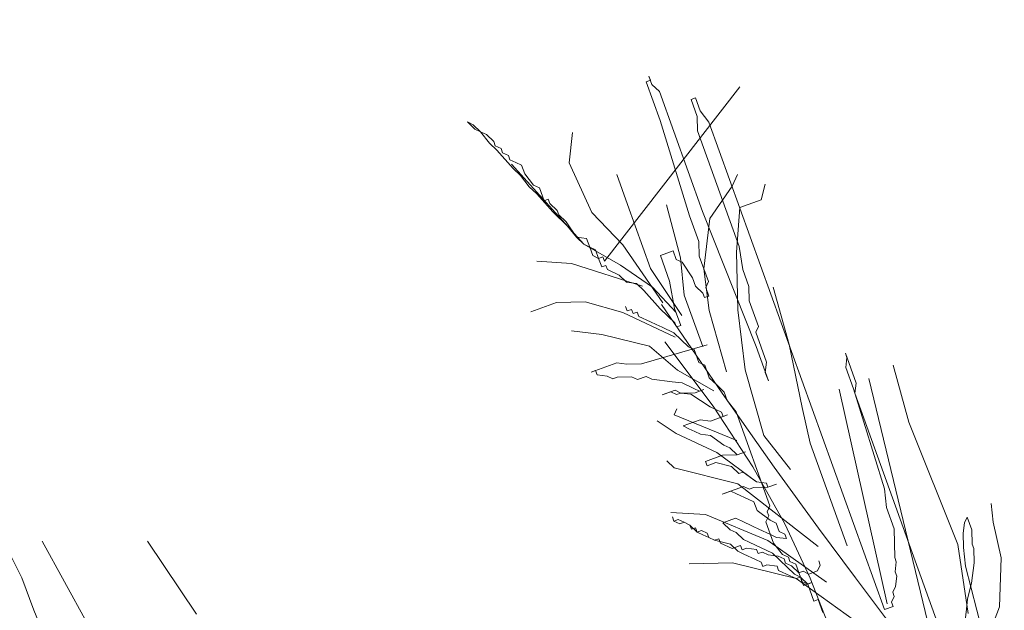
# Model space of a CAD drawing. Units: millimetres. Extents: x 595116 to 630915, y 909473 to 920225.
# Tile 88 of 134: x 629714.705 to 629720.901, y 919281.384 to 919285.103. Entities that reach past the tile are written whole.
import ezdxf

# ---------------------------------------------------------------- set-up
doc = ezdxf.new("R2010")
doc.units = ezdxf.units.MM
doc.layers.add('Dimension', color=3, linetype='Continuous', lineweight=18)
doc.layers.add('L-PLNT', color=85, linetype='Continuous', lineweight=13)
doc.styles.get("Standard").update_dxf_attribs({"font": 'arial.ttf'})
doc.dimstyles.new('ISO-25', dxfattribs={"dimtxt": 9, "dimasz": 6, "dimexe": 1.25, "dimexo": 0.625, "dimtad": 1, "dimlunit": 4, "dimtxsty": 'Standard', "dimcen": 2.5, "dimadec": 0, "dimazin": 0, "dimtfac": 1, "dimtmove": 0, "dimatfit": 3, "dimfxl": 1, "dimarcsym": 0})

# ---------------------------------------------------------------- blocks, each defined once
blk = doc.blocks.new('A$C4FB75ABC')
for p, q in [((2.238, 4.7104), (2.2329, 4.7248)), ((2.2329, 4.7248), (2.2354, 4.7176)), ((2.1583, 4.4143), (2.3852, 4.7066)), ((2.2354, 4.7176), (2.2283, 4.715)), ((2.2283, 4.715), (2.2515, 4.6504)), ((2.2504, 4.6987), (2.238, 4.7104)), ((2.3227, 4.4977), (2.2504, 4.6987)), ((2.3109, 4.688), (2.3037, 4.6854)), ((2.3037, 4.6854), (2.314, 4.6567)), ((2.3186, 4.6665), (2.3109, 4.688)), ((2.314, 4.6567), (2.3146, 4.6326)), ((2.3336, 4.6475), (2.3186, 4.6665)), ((1.9382, 4.6431), (1.9285, 4.6477)), ((1.9285, 4.6477), (1.9408, 4.6359)), ((1.9506, 4.6313), (1.9382, 4.6431)), ((2.2515, 4.6504), (2.3011, 4.49)), ((2.6279, 3.8295), (2.3336, 4.6475)), ((1.9408, 4.6359), (1.9506, 4.6313)), ((1.9603, 4.6267), (1.9506, 4.6313)), ((1.9506, 4.6313), (1.9655, 4.6124)), ((1.9726, 4.6149), (1.9603, 4.6267)), ((2.0989, 4.5793), (2.1049, 4.6301)), ((2.3146, 4.6326), (2.3843, 4.4389)), ((1.9655, 4.6124), (1.9778, 4.6006)), ((1.9752, 4.6078), (1.9726, 4.6149)), ((1.985, 4.6032), (1.9752, 4.6078)), ((1.9778, 4.6006), (2.0051, 4.5699)), ((1.9876, 4.596), (1.985, 4.6032)), ((1.9973, 4.5914), (1.9876, 4.596)), ((1.9999, 4.5842), (1.9973, 4.5914)), ((2.0097, 4.5796), (1.9999, 4.5842)), ((2.1238, 4.4424), (2.0025, 4.577)), ((2.0194, 4.575), (2.0097, 4.5796)), ((2.0246, 4.5607), (2.0194, 4.575)), ((2.137, 4.4958), (2.0989, 4.5793)), ((2.0051, 4.5699), (2.0174, 4.5581)), ((2.0174, 4.5581), (2.0323, 4.5391)), ((2.0395, 4.5417), (2.0246, 4.5607)), ((2.197, 4.5092), (2.1789, 4.5595)), ((2.3723, 4.5399), (2.3815, 4.5594)), ((2.0493, 4.5371), (2.0395, 4.5417)), ((2.4211, 4.5169), (2.4277, 4.5436)), ((2.0323, 4.5391), (2.0447, 4.5274)), ((2.0447, 4.5274), (2.0719, 4.4967)), ((2.057, 4.5156), (2.0493, 4.5371)), ((2.335, 4.486), (2.3723, 4.5399)), ((2.0642, 4.5182), (2.057, 4.5156)), ((2.0668, 4.511), (2.0642, 4.5182)), ((2.0791, 4.4992), (2.0668, 4.511)), ((2.2357, 4.4016), (2.197, 4.5092)), ((2.2859, 4.4197), (2.2621, 4.5084)), ((2.3852, 4.504), (2.4211, 4.5169)), ((2.0719, 4.4967), (2.0966, 4.4731)), ((2.0817, 4.4921), (2.0791, 4.4992)), ((2.094, 4.4803), (2.0817, 4.4921)), ((2.189, 4.4415), (2.137, 4.4958)), ((2.4125, 4.2707), (2.3227, 4.4977)), ((2.3797, 4.4291), (2.3852, 4.504)), ((2.1115, 4.4542), (2.094, 4.4803)), ((2.3011, 4.49), (2.3166, 4.4469)), ((2.325, 4.4013), (2.335, 4.486)), ((2.0966, 4.4731), (2.1115, 4.4542)), ((2.1238, 4.4424), (2.1115, 4.4542)), ((2.1115, 4.4542), (2.1284, 4.4522)), ((2.1336, 4.4378), (2.1238, 4.4424)), ((2.185, 4.4077), (2.1238, 4.4424)), ((2.1284, 4.4522), (2.1336, 4.4378)), ((2.2564, 4.3442), (2.189, 4.4415)), ((2.3166, 4.4469), (2.3172, 4.4228)), ((2.1388, 4.4235), (2.1336, 4.4378)), ((2.1336, 4.4378), (2.1434, 4.4332)), ((2.1434, 4.4332), (2.1485, 4.4189)), ((2.2736, 4.4314), (2.2521, 4.4237)), ((2.2788, 4.4171), (2.2736, 4.4314)), ((2.382, 4.3327), (2.3797, 4.4291)), ((2.3843, 4.4389), (2.3901, 4.4004)), ((2.1029, 4.4105), (2.0449, 4.414)), ((2.222, 4.3723), (2.1029, 4.4105)), ((2.1485, 4.4189), (2.1388, 4.4235)), ((2.1485, 4.4189), (2.1557, 4.4214)), ((2.1537, 4.4045), (2.1485, 4.4189)), ((2.1557, 4.4214), (2.1583, 4.4143)), ((2.2521, 4.4237), (2.2676, 4.3807)), ((2.2885, 4.4125), (2.2788, 4.4171)), ((2.2922, 4.3571), (2.2859, 4.4197)), ((2.306, 4.3864), (2.2885, 4.4125)), ((2.3172, 4.4228), (2.3327, 4.3798)), ((2.1609, 4.4071), (2.1537, 4.4045)), ((2.1634, 4.3999), (2.1609, 4.4071)), ((2.1829, 4.3907), (2.1634, 4.3999)), ((2.2389, 4.3703), (2.185, 4.4077)), ((2.2882, 4.3232), (2.2357, 4.4016)), ((2.3338, 4.3316), (2.325, 4.4013)), ((2.3901, 4.4004), (2.4004, 4.3717)), ((2.1953, 4.379), (2.1829, 4.3907)), ((2.2122, 4.3769), (2.1953, 4.379)), ((2.2245, 4.3652), (2.2122, 4.3769)), ((2.2676, 4.3807), (2.2759, 4.335)), ((2.3112, 4.372), (2.306, 4.3864)), ((2.3327, 4.3798), (2.3281, 4.37)), ((2.2518, 4.3344), (2.2245, 4.3652)), ((2.2785, 4.3278), (2.2389, 4.3703)), ((2.3235, 4.3603), (2.3112, 4.372)), ((2.3261, 4.3531), (2.3235, 4.3603)), ((2.3281, 4.37), (2.3333, 4.3557)), ((2.4004, 4.3717), (2.401, 4.3476)), ((2.4678, 4.2744), (2.4414, 4.3703)), ((2.0779, 4.3448), (2.0349, 4.3293)), ((2.1261, 4.346), (2.0779, 4.3448)), ((2.1893, 4.3282), (2.1261, 4.346)), ((2.3232, 4.271), (2.2922, 4.3571)), ((2.3333, 4.3557), (2.3261, 4.3531)), ((2.401, 4.3476), (2.4165, 4.3046)), ((2.277, 4.2868), (2.1893, 4.3282)), ((2.1938, 4.3379), (2.1964, 4.3307)), ((2.1964, 4.3307), (2.2036, 4.3333)), ((2.2036, 4.3333), (2.2062, 4.3261)), ((2.2062, 4.3261), (2.2134, 4.3287)), ((2.2134, 4.3287), (2.2159, 4.3215)), ((2.2641, 4.3227), (2.2518, 4.3344)), ((2.2538, 4.3417), (2.3557, 4.1924)), ((2.2759, 4.335), (2.2862, 4.3063)), ((2.3628, 4.2285), (2.3338, 4.3316)), ((2.3941, 4.2317), (2.382, 4.3327)), ((2.2159, 4.3215), (2.2354, 4.3124)), ((2.2354, 4.3124), (2.2452, 4.3078)), ((2.2765, 4.3109), (2.2641, 4.3227)), ((2.2791, 4.3037), (2.2765, 4.3109)), ((2.154, 4.2911), (2.1032, 4.2972)), ((2.2452, 4.3078), (2.255, 4.3032)), ((2.255, 4.3032), (2.2745, 4.294)), ((2.2745, 4.294), (2.2868, 4.2822)), ((2.2862, 4.3063), (2.2791, 4.3037)), ((2.4165, 4.3046), (2.4119, 4.2948)), ((2.4119, 4.2948), (2.43, 4.2446)), ((2.234, 4.2713), (2.154, 4.2911)), ((2.3407, 4.1707), (2.2593, 4.2788)), ((2.2868, 4.2822), (2.2991, 4.2704)), ((2.2202, 4.242), (2.3304, 4.2736)), ((2.2808, 4.2314), (2.234, 4.2713)), ((2.2991, 4.2704), (2.3089, 4.2658)), ((2.3089, 4.2658), (2.3166, 4.2443)), ((2.4331, 4.2133), (2.4125, 4.2707)), ((2.4896, 4.1688), (2.4678, 4.2744)), ((2.5803, 4.2095), (2.5622, 4.2597)), ((2.5622, 4.2597), (2.5648, 4.2526)), ((2.1362, 4.228), (2.1792, 4.2435)), ((2.1792, 4.2435), (2.1961, 4.2415)), ((2.3166, 4.2443), (2.3264, 4.2397)), ((2.43, 4.2446), (2.4279, 4.2276)), ((2.5648, 4.2526), (2.5628, 4.2356)), ((2.1434, 4.2306), (2.1362, 4.228)), ((2.1459, 4.2234), (2.1434, 4.2306)), ((2.1961, 4.2415), (2.2202, 4.242)), ((2.3419, 4.1967), (2.2808, 4.2314)), ((2.3264, 4.2397), (2.3341, 4.2182)), ((2.4257, 4.1214), (2.3941, 4.2317)), ((2.4279, 4.2276), (2.4331, 4.2133)), ((2.5628, 4.2356), (2.5757, 4.1997)), ((2.6686, 4.144), (2.6423, 4.2399)), ((2.1629, 4.2214), (2.1459, 4.2234)), ((2.1726, 4.2168), (2.1629, 4.2214)), ((2.1798, 4.2194), (2.1726, 4.2168)), ((2.2039, 4.22), (2.1798, 4.2194)), ((2.2136, 4.2154), (2.2039, 4.22)), ((2.228, 4.2205), (2.2136, 4.2154)), ((2.2377, 4.2159), (2.228, 4.2205)), ((2.2716, 4.2119), (2.2377, 4.2159)), ((2.2885, 4.2099), (2.2716, 4.2119)), ((2.308, 4.2007), (2.2885, 4.2099)), ((2.3341, 4.2182), (2.3465, 4.2064)), ((2.7169, 3.7399), (2.6018, 4.2172)), ((2.2552, 4.1898), (2.2768, 4.1975)), ((2.2696, 4.195), (2.2552, 4.1898)), ((2.2793, 4.1904), (2.2696, 4.195)), ((2.2768, 4.1975), (2.2865, 4.1929)), ((2.2865, 4.1929), (2.3106, 4.1935)), ((2.3178, 4.1961), (2.308, 4.2007)), ((2.3106, 4.1935), (2.325, 4.1987)), ((2.325, 4.1987), (2.3178, 4.1961)), ((2.3465, 4.2064), (2.3588, 4.1946)), ((2.3588, 4.1946), (2.364, 4.1803)), ((2.6325, 3.8393), (2.5516, 4.1992)), ((2.5757, 4.1997), (2.6279, 4.0321)), ((2.5783, 4.1926), (2.5803, 4.2095)), ((2.2865, 4.1929), (2.2793, 4.1904)), ((2.3034, 4.1909), (2.2865, 4.1929)), ((2.3353, 4.17), (2.3034, 4.1909)), ((2.3557, 4.1924), (2.443, 4.0685)), ((2.364, 4.1803), (2.3789, 4.1614)), ((2.8029, 3.5683), (2.5783, 4.1926)), ((2.2753, 4.1565), (2.2799, 4.1663)), ((2.345, 4.1654), (2.3353, 4.17)), ((2.4072, 4.0691), (2.3407, 4.1707)), ((2.3548, 4.1608), (2.345, 4.1654)), ((2.3574, 4.1536), (2.3548, 4.1608)), ((2.3789, 4.1614), (2.4357, 4.0035)), ((2.5031, 4.1088), (2.4896, 4.1688)), ((2.2785, 4.1252), (2.2466, 4.1462)), ((2.38, 4.1131), (2.2753, 4.1565)), ((2.2902, 4.1376), (2.3189, 4.1479)), ((2.3189, 4.1479), (2.3359, 4.1459)), ((2.3359, 4.1459), (2.3645, 4.1562)), ((2.3645, 4.1562), (2.3574, 4.1536)), ((2.7507, 3.9385), (2.6686, 4.144)), ((2.3, 4.133), (2.2902, 4.1376)), ((2.3098, 4.1284), (2.3, 4.133)), ((2.3195, 4.1238), (2.3098, 4.1284)), ((2.3468, 4.0931), (2.2785, 4.1252)), ((2.3364, 4.1218), (2.3195, 4.1238)), ((2.3585, 4.1054), (2.3364, 4.1218)), ((2.4704, 4.0646), (2.4257, 4.1214)), ((2.3683, 4.1008), (2.3585, 4.1054)), ((2.3806, 4.089), (2.3683, 4.1008)), ((2.5651, 3.9366), (2.5031, 4.1088)), ((2.275, 4.0672), (2.2627, 4.079)), ((2.3278, 4.0781), (2.3565, 4.0885)), ((2.3304, 4.071), (2.3278, 4.0781)), ((2.413, 4.044), (2.3468, 4.0931)), ((2.3565, 4.0885), (2.3806, 4.089)), ((2.3806, 4.089), (2.395, 4.0942)), ((2.395, 4.0942), (2.3806, 4.089)), ((2.3818, 4.0408), (2.275, 4.0672)), ((2.3448, 4.0761), (2.3304, 4.071)), ((2.3714, 4.0695), (2.3448, 4.0761)), ((2.3838, 4.0577), (2.3714, 4.0695)), ((2.4608, 3.9732), (2.4072, 4.0691)), ((2.443, 4.0685), (2.5171, 3.9664)), ((2.3909, 4.0603), (2.3838, 4.0577)), ((2.413, 4.044), (2.3909, 4.0603)), ((2.3557, 4.0233), (2.3915, 4.0362)), ((2.37, 4.0285), (2.3557, 4.0233)), ((2.3798, 4.0239), (2.37, 4.0285)), ((2.5169, 3.9354), (2.3818, 4.0408)), ((2.3915, 4.0362), (2.4013, 4.0316)), ((2.4013, 4.0316), (2.4084, 4.0342)), ((2.4084, 4.0342), (2.4325, 4.0348)), ((2.43, 4.0419), (2.413, 4.044)), ((2.4325, 4.0348), (2.43, 4.0419)), ((2.4325, 4.0348), (2.4469, 4.0399)), ((2.4469, 4.0399), (2.4325, 4.0348)), ((2.6279, 4.0321), (2.6311, 4.0008)), ((2.3993, 4.0147), (2.3798, 4.0239)), ((2.409, 4.0101), (2.3993, 4.0147)), ((2.4142, 3.9957), (2.409, 4.0101)), ((2.4363, 3.9794), (2.4142, 3.9957)), ((2.4357, 4.0035), (2.4311, 3.9937)), ((2.6311, 4.0008), (2.644, 3.965)), ((2.8101, 3.9761), (2.8069, 4.0074)), ((2.3275, 3.9889), (2.2696, 3.9923)), ((2.2748, 3.978), (2.2722, 3.9852)), ((2.2722, 3.9852), (2.2748, 3.978)), ((2.2748, 3.978), (2.2819, 3.9806)), ((2.2819, 3.9806), (2.2917, 3.976)), ((2.4323, 3.9455), (2.3275, 3.9889)), ((2.3568, 3.9751), (2.3783, 3.9828)), ((2.3783, 3.9828), (2.3881, 3.9782)), ((2.4337, 3.9866), (2.4291, 3.9768)), ((2.4311, 3.9937), (2.4337, 3.9866)), ((2.446, 3.9748), (2.4363, 3.9794)), ((2.7665, 3.9847), (2.7619, 3.975)), ((2.7742, 3.9632), (2.7665, 3.9847)), ((2.2845, 3.9734), (2.2748, 3.978)), ((2.2917, 3.976), (2.2845, 3.9734)), ((2.3014, 3.9714), (2.2917, 3.976)), ((2.2917, 3.976), (2.3014, 3.9714)), ((2.304, 3.9642), (2.3014, 3.9714)), ((2.3014, 3.9714), (2.3138, 3.9596)), ((2.3112, 3.9668), (2.304, 3.9642)), ((2.3138, 3.9596), (2.3112, 3.9668)), ((2.3691, 3.9633), (2.3568, 3.9751)), ((2.3789, 3.9587), (2.3691, 3.9633)), ((2.3881, 3.9782), (2.4076, 3.9691)), ((2.4076, 3.9691), (2.4173, 3.9645)), ((2.4173, 3.9645), (2.4368, 3.9553)), ((2.4291, 3.9768), (2.442, 3.9409)), ((2.4512, 3.9604), (2.446, 3.9748)), ((2.5035, 3.8821), (2.4608, 3.9732)), ((2.5171, 3.9664), (2.5794, 3.8826)), ((2.644, 3.965), (2.6451, 3.9167)), ((2.7619, 3.975), (2.7599, 3.958)), ((2.7748, 3.9391), (2.7742, 3.9632)), ((2.8236, 3.9161), (2.8101, 3.9761)), ((2.3209, 3.9622), (2.3138, 3.9596)), ((2.3138, 3.9596), (2.3235, 3.955)), ((2.3307, 3.9576), (2.3209, 3.9622)), ((2.3235, 3.955), (2.3333, 3.9504)), ((2.3333, 3.9504), (2.3307, 3.9576)), ((2.343, 3.9458), (2.3333, 3.9504)), ((2.3333, 3.9504), (2.343, 3.9458)), ((2.3502, 3.9484), (2.343, 3.9458)), ((2.343, 3.9458), (2.3697, 3.9392)), ((2.3528, 3.9412), (2.3502, 3.9484)), ((2.3912, 3.947), (2.3789, 3.9587)), ((2.401, 3.9424), (2.3912, 3.947)), ((2.4368, 3.9553), (2.4466, 3.9507)), ((2.4466, 3.9507), (2.4635, 3.9487)), ((2.4609, 3.9558), (2.4512, 3.9604)), ((2.4635, 3.9487), (2.4609, 3.9558)), ((2.7599, 3.958), (2.7605, 3.9339)), ((1.154, 3.9374), (1.1812, 3.8829)), ((1.2153, 3.9442), (1.2902, 3.808)), ((1.3924, 3.9442), (1.4742, 3.8217)), ((2.3723, 3.932), (2.3528, 3.9412)), ((2.3697, 3.9392), (2.3821, 3.9274)), ((2.3866, 3.9372), (2.3723, 3.932)), ((2.3892, 3.93), (2.3866, 3.9372)), ((2.3964, 3.9326), (2.3892, 3.93)), ((2.4133, 3.9306), (2.3964, 3.9326)), ((2.44, 3.924), (2.401, 3.9424)), ((2.4159, 3.9234), (2.4133, 3.9306)), ((2.5304, 3.8755), (2.4323, 3.9455)), ((2.442, 3.9409), (2.4569, 3.922)), ((2.7679, 3.8231), (2.7507, 3.9385)), ((2.7605, 3.9339), (2.7636, 3.9026)), ((2.7774, 3.9319), (2.7748, 3.9391)), ((2.778, 3.9078), (2.7774, 3.9319)), ((2.3821, 3.9274), (2.3918, 3.9228)), ((2.3918, 3.9228), (2.4113, 3.9137)), ((2.4113, 3.9137), (2.4211, 3.9091)), ((2.4231, 3.926), (2.4159, 3.9234)), ((2.4328, 3.9214), (2.4231, 3.926)), ((2.4498, 3.9194), (2.4328, 3.9214)), ((2.4523, 3.9122), (2.44, 3.924)), ((2.4595, 3.9148), (2.4498, 3.9194)), ((2.4569, 3.922), (2.4667, 3.9174)), ((2.4621, 3.9076), (2.4595, 3.9148)), ((2.4667, 3.9174), (2.4693, 3.9102)), ((2.6451, 3.9167), (2.6477, 3.9096)), ((2.8207, 3.834), (2.8236, 3.9161)), ((2.3729, 3.9079), (2.3006, 3.9062)), ((2.4796, 3.8815), (2.3729, 3.9079)), ((2.4211, 3.9091), (2.4237, 3.9019)), ((2.4237, 3.9019), (2.4308, 3.9045)), ((2.4308, 3.9045), (2.4478, 3.9025)), ((2.4478, 3.9025), (2.4503, 3.8953)), ((2.477, 3.8887), (2.4523, 3.9122)), ((2.4718, 3.903), (2.4621, 3.9076)), ((2.4693, 3.9102), (2.479, 3.9056)), ((2.4842, 3.8913), (2.4718, 3.903)), ((2.479, 3.9056), (2.4868, 3.8841)), ((2.52, 3.9042), (2.5155, 3.8944)), ((2.5175, 3.9113), (2.52, 3.9042)), ((2.6477, 3.9096), (2.6457, 3.8926)), ((2.7636, 3.9026), (2.8247, 3.6653)), ((2.7739, 3.8739), (2.778, 3.9078)), ((1.1812, 3.8829), (1.2017, 3.8285)), ((2.4503, 3.8953), (2.4698, 3.8861)), ((2.4698, 3.8861), (2.4796, 3.8815)), ((2.4868, 3.8841), (2.477, 3.8887)), ((2.4796, 3.8815), (2.4868, 3.8841)), ((2.5777, 3.8114), (2.4796, 3.8815)), ((2.4914, 3.8938), (2.4842, 3.8913)), ((2.4868, 3.8841), (2.4893, 3.8769)), ((2.4919, 3.8697), (2.4868, 3.8841)), ((2.4868, 3.8841), (2.4991, 3.8723)), ((2.5011, 3.8892), (2.4914, 3.8938)), ((2.5155, 3.8944), (2.5011, 3.8892)), ((2.5372, 3.7949), (2.5035, 3.8821)), ((2.5794, 3.8826), (2.6314, 3.8136)), ((2.6457, 3.8926), (2.6483, 3.8855)), ((2.6483, 3.8855), (2.6463, 3.8685)), ((2.4893, 3.8769), (2.4991, 3.8723)), ((2.5063, 3.8749), (2.4919, 3.8697)), ((2.4991, 3.8723), (2.5063, 3.8749)), ((2.4991, 3.8723), (2.5094, 3.8436)), ((2.6463, 3.8685), (2.6417, 3.8588)), ((2.7673, 3.8473), (2.7739, 3.8739)), ((2.6443, 3.8516), (2.6397, 3.8418)), ((2.6417, 3.8588), (2.6443, 3.8516)), ((2.7653, 3.8303), (2.7673, 3.8473)), ((2.5094, 3.8436), (2.5166, 3.8462)), ((2.5166, 3.8462), (2.5244, 3.8247)), ((2.6423, 3.8347), (2.6279, 3.8295)), ((2.6397, 3.8418), (2.6423, 3.8347)), ((2.7613, 3.7965), (2.7653, 3.8303)), ((2.7957, 3.7683), (2.8207, 3.834)), ((1.2017, 3.8285), (1.2153, 3.7944))]:
    blk.add_line(p, q)
blk = doc.blocks.new('*D216')
at = {"layer": 'Defpoints', "color": 0, "transparency": 16777216}
for p in [(629743.5408, 919411.9276), (629505.0408, 919411.8279), (629743.5408, 918832.3776)]:
    blk.add_point(p, dxfattribs=at)
at = {"layer": 'Dimension', "color": 0, "lineweight": -2, "transparency": 16777216}
for p, q in [((629743.5408, 919411.3026), (629743.5408, 918831.1276)), ((629505.0408, 919411.2029), (629505.0408, 918831.1276)), ((629511.0408, 918832.3776), (629737.5408, 918832.3776))]:
    blk.add_line(p, q, dxfattribs=at)
at = {"layer": 'Dimension', "color": 0, "transparency": 16777216}
for points in [[(629511.0408, 918833.3776), (629511.0408, 918831.3776), (629505.0408, 918832.3776)], [(629737.5408, 918833.3776), (629737.5408, 918831.3776), (629743.5408, 918832.3776)]]:
    blk.add_solid(points, dxfattribs=at)
at = {"layer": 'Dimension', "color": 0, "transparency": 16777216, "insert": (629624.2908, 918837.656), "char_height": 9, "attachment_point": 5}
blk.add_mtext('19\'-10 1/2"', dxfattribs=at)

msp = doc.modelspace()

# ---------------------------------------------------------------- block references
at = {"layer": 'L-PLNT', "xscale": 3.753413438031968, "yscale": 3.753413438031968, "zscale": 3.753413438031968}
msp.add_blockref('A$C4FB75ABC', (629710.2837, 919267.0144), dxfattribs=at)

# ---------------------------------------------------------------- dimensions: what is measured, and where the dimension line sits
at = {"layer": 'Dimension'}
dim = msp.add_linear_dim(base=(629743.5408, 918832.3776), p1=(629505.0408, 919411.8279), p2=(629743.5408, 919411.9276), dimstyle='ISO-25', override={"dimdec": 1, "dimlfac": 1, "dimrnd": 0, "dimzin": 1, "dimdsep": 46, "dimlunit": 4, "dimfrac": 2}, dxfattribs=at)
dim.commit()
dim.dimension.update_dxf_attribs({"geometry": '*D216', "text_midpoint": (629624.2908, 918837.656)})

doc.saveas('drawing.dxf')
